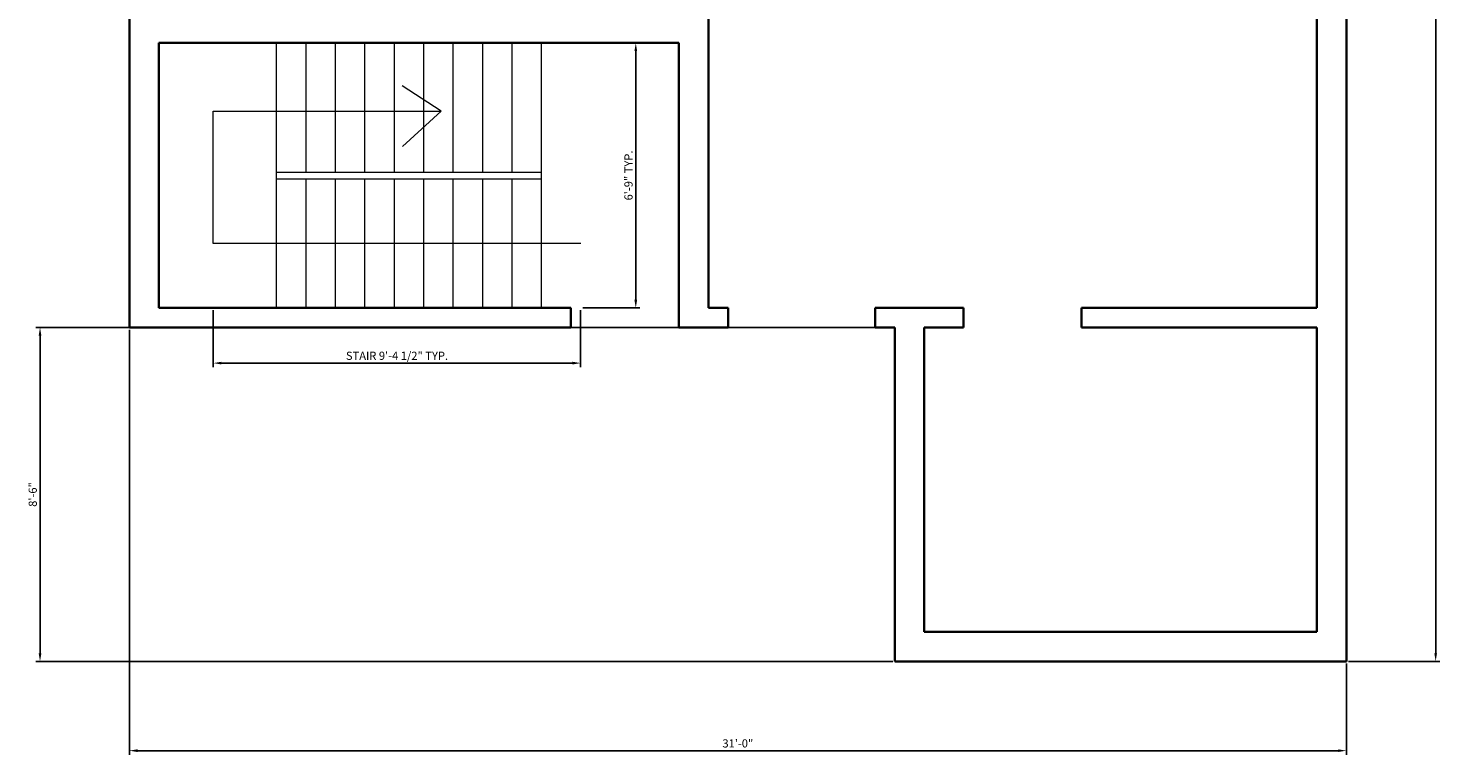
# Model space of a CAD drawing. Units: inches. Extents: x 2163 to 7246, y 928 to 2098.
# Tile 14 of 15: x 6815 to 7246, y 1403 to 1625. Entities that reach past the tile are written whole.
import ezdxf

# ---------------------------------------------------------------- set-up
doc = ezdxf.new("R2010")
doc.units = ezdxf.units.IN
for name, color, linetype, lineweight in [('A-ANNO-DIMS', 4, 'Continuous', 18), ('A-FLOR-STRS', 7, 'Continuous', 20), ('A-WALL', 7, 'Continuous', 35)]:
    doc.layers.add(name, color=color, linetype=linetype, lineweight=lineweight)
doc.styles.get("Standard").update_dxf_attribs({"font": 'arial.ttf'})
doc.dimstyles.new('ISO-25', dxfattribs={"dimtxt": 2.5, "dimasz": 2.5, "dimexe": 1.25, "dimexo": 0.625, "dimtad": 1, "dimdec": 0, "dimlunit": 3, "dimtxsty": 'Standard', "dimcen": 2.5, "dimadec": 0, "dimazin": 0, "dimtfac": 1, "dimtdec": 0, "dimtmove": 0, "dimatfit": 3, "dimfxl": 1, "dimarcsym": 0})

# ---------------------------------------------------------------- blocks, each defined once
blk = doc.blocks.new('STAIR-DOGLEG-81')
for p, q in [((19.35, 0), (19.35, 81)), ((28.35, 41.5), (28.35, 81)), ((37.35, 41.5), (37.35, 81)), ((46.35, 41.5), (46.35, 81)), ((55.35, 41.5), (55.35, 81)), ((64.35, 41.5), (64.35, 81)), ((73.35, 41.5), (73.35, 81)), ((82.35, 41.5), (82.35, 81)), ((91.35, 41.5), (91.35, 81)), ((100.35, 0), (100.35, 81)), ((69.69, 60.16), (57.76, 67.88)), ((0, 19.75), (0, 60.16)), ((0, 60.16), (69.69, 60.16)), ((69.69, 60.16), (57.82, 49.34)), ((19.35, 41.5), (100.35, 41.5)), ((19.35, 39.5), (100.35, 39.5)), ((28.35, 0), (28.35, 39.5)), ((37.35, 0), (37.35, 39.5)), ((46.35, 0), (46.35, 39.5)), ((55.35, 0), (55.35, 39.5)), ((64.35, 0), (64.35, 39.5)), ((73.35, 0), (73.35, 39.5)), ((82.35, 0), (82.35, 39.5)), ((91.35, 0), (91.35, 39.5)), ((112.3, 19.75), (0, 19.75))]:
    blk.add_line(p, q)
blk = doc.blocks.new('*D69')
at = {"layer": 'A-ANNO-DIMS', "color": 0, "lineweight": -2, "transparency": 16777216}
for p, q in [((6871.12, 1538.83), (6871.12, 1521.36)), ((6983.41, 1538.83), (6983.41, 1521.36)), ((6873.62, 1522.61), (6980.91, 1522.61))]:
    blk.add_line(p, q, dxfattribs=at)
at = {"layer": 'A-ANNO-DIMS', "color": 0, "transparency": 16777216}
for points in [[(6873.62, 1523.03), (6873.62, 1522.2), (6871.12, 1522.61)], [(6980.91, 1523.03), (6980.91, 1522.2), (6983.41, 1522.61)]]:
    blk.add_solid(points, dxfattribs=at)
at = {"layer": 'Defpoints', "color": 0, "transparency": 16777216}
for p in [(6871.12, 1539.46), (6983.41, 1539.46), (6983.41, 1522.61)]:
    blk.add_point(p, dxfattribs=at)
at = {"layer": 'A-ANNO-DIMS', "color": 0, "transparency": 16777216, "insert": (6927.27, 1524.53), "char_height": 2.5, "attachment_point": 5}
blk.add_mtext('STAIR 9\'-4 1/2" TYP.', dxfattribs=at)
blk = doc.blocks.new('*D70')
at = {"layer": 'A-ANNO-DIMS', "color": 0, "lineweight": -2, "transparency": 16777216}
for p, q in [((6984.04, 1620.46), (7001.51, 1620.46)), ((7000.26, 1541.96), (7000.26, 1617.96)), ((6984.04, 1539.46), (7001.51, 1539.46))]:
    blk.add_line(p, q, dxfattribs=at)
at = {"layer": 'A-ANNO-DIMS', "color": 0, "transparency": 16777216}
for points in [[(6999.84, 1617.96), (7000.68, 1617.96), (7000.26, 1620.46)], [(6999.84, 1541.96), (7000.68, 1541.96), (7000.26, 1539.46)]]:
    blk.add_solid(points, dxfattribs=at)
at = {"layer": 'Defpoints', "color": 0, "transparency": 16777216}
for p in [(6983.41, 1620.46), (7000.26, 1620.46), (6983.41, 1539.46)]:
    blk.add_point(p, dxfattribs=at)
at = {"layer": 'A-ANNO-DIMS', "color": 0, "transparency": 16777216, "insert": (6998.36, 1579.96), "char_height": 2.5, "attachment_point": 5, "rotation": 90}
blk.add_mtext('6\'-9" TYP.', dxfattribs=at)
blk = doc.blocks.new('*D112')
at = {"layer": 'A-ANNO-DIMS', "color": 0, "lineweight": -2, "transparency": 16777216}
for p, q in [((6845.46, 1532.83), (6845.46, 1402.91)), ((7217.46, 1430.83), (7217.46, 1402.91)), ((6847.96, 1404.16), (7214.96, 1404.16))]:
    blk.add_line(p, q, dxfattribs=at)
at = {"layer": 'A-ANNO-DIMS', "color": 0, "transparency": 16777216}
for points in [[(6847.96, 1404.58), (6847.96, 1403.74), (6845.46, 1404.16)], [(7214.96, 1404.58), (7214.96, 1403.74), (7217.46, 1404.16)]]:
    blk.add_solid(points, dxfattribs=at)
at = {"layer": 'Defpoints', "color": 0, "transparency": 16777216}
for p in [(6845.46, 1533.46), (7217.46, 1431.46), (7217.46, 1404.16)]:
    blk.add_point(p, dxfattribs=at)
at = {"layer": 'A-ANNO-DIMS', "color": 0, "transparency": 16777216, "insert": (7031.46, 1406.06), "char_height": 2.5, "attachment_point": 5}
blk.add_mtext('31\'-0"', dxfattribs=at)
blk = doc.blocks.new('*D113')
at = {"layer": 'A-ANNO-DIMS', "color": 0, "lineweight": -2, "transparency": 16777216}
for p, q in [((7218.09, 1974.46), (7246.01, 1974.46)), ((7244.76, 1971.96), (7244.76, 1433.96)), ((7218.09, 1431.46), (7246.01, 1431.46))]:
    blk.add_line(p, q, dxfattribs=at)
at = {"layer": 'A-ANNO-DIMS', "color": 0, "transparency": 16777216}
for points in [[(7244.34, 1971.96), (7245.18, 1971.96), (7244.76, 1974.46)], [(7244.34, 1433.96), (7245.18, 1433.96), (7244.76, 1431.46)]]:
    blk.add_solid(points, dxfattribs=at)
at = {"layer": 'Defpoints', "color": 0, "transparency": 16777216}
for p in [(7217.46, 1974.46), (7217.46, 1431.46), (7244.76, 1431.46)]:
    blk.add_point(p, dxfattribs=at)
at = {"layer": 'A-ANNO-DIMS', "color": 0, "transparency": 16777216, "insert": (7242.86, 1702.96), "char_height": 2.5, "attachment_point": 5, "rotation": 90}
blk.add_mtext('45\'-3"', dxfattribs=at)
blk = doc.blocks.new('*D114')
at = {"layer": 'A-ANNO-DIMS', "color": 0, "lineweight": -2, "transparency": 16777216}
for p, q in [((7078.84, 1533.46), (6816.91, 1533.46)), ((6818.16, 1530.96), (6818.16, 1433.96)), ((7078.84, 1431.46), (6816.91, 1431.46))]:
    blk.add_line(p, q, dxfattribs=at)
at = {"layer": 'A-ANNO-DIMS', "color": 0, "transparency": 16777216}
for points in [[(6817.74, 1530.96), (6818.58, 1530.96), (6818.16, 1533.46)], [(6817.74, 1433.96), (6818.58, 1433.96), (6818.16, 1431.46)]]:
    blk.add_solid(points, dxfattribs=at)
at = {"layer": 'Defpoints', "color": 0, "transparency": 16777216}
for p in [(7079.46, 1533.46), (6818.16, 1431.46), (7079.46, 1431.46)]:
    blk.add_point(p, dxfattribs=at)
at = {"layer": 'A-ANNO-DIMS', "color": 0, "transparency": 16777216, "insert": (6816.26, 1482.46), "char_height": 2.5, "attachment_point": 5, "rotation": 90}
blk.add_mtext('8\'-6"', dxfattribs=at)

msp = doc.modelspace()

# ---------------------------------------------------------------- linework, layer by layer
at = {"layer": 'A-WALL'}
for p, q in [((6845.46, 1533.46), (6845.46, 1974.46)), ((7217.46, 1974.46), (7217.46, 1431.46)), ((7208.46, 1815.46), (7208.46, 1539.46)), ((7022.46, 1755.46), (7022.46, 1539.46)), ((6854.46, 1620.46), (7013.46, 1620.46)), ((6854.46, 1539.46), (6854.46, 1620.46)), ((7013.46, 1620.46), (7013.46, 1533.46)), ((6854.46, 1539.46), (6980.46, 1539.46)), ((6980.46, 1533.46), (6980.46, 1539.46)), ((7022.46, 1539.46), (7028.46, 1539.46)), ((7028.46, 1539.46), (7028.46, 1533.46)), ((7073.46, 1539.46), (7100.46, 1539.46)), ((7073.46, 1539.46), (7073.46, 1533.46)), ((7100.46, 1539.46), (7100.46, 1533.46)), ((7136.46, 1539.46), (7208.46, 1539.46)), ((7136.46, 1539.46), (7136.46, 1533.46)), ((6845.46, 1533.46), (6980.46, 1533.46)), ((7013.46, 1533.46), (7028.46, 1533.46)), ((7073.46, 1533.46), (7079.46, 1533.46)), ((7079.46, 1533.46), (7079.46, 1431.46)), ((7088.46, 1533.46), (7100.46, 1533.46)), ((7088.46, 1533.46), (7088.46, 1440.46)), ((7136.46, 1533.46), (7208.46, 1533.46)), ((7208.46, 1533.46), (7208.46, 1440.46)), ((7208.46, 1440.46), (7088.46, 1440.46)), ((7217.46, 1431.46), (7079.46, 1431.46))]:
    msp.add_line(p, q, dxfattribs=at)

# ---------------------------------------------------------------- block references
at = {"layer": 'A-FLOR-STRS'}
msp.add_blockref('STAIR-DOGLEG-81', (6871.12, 1539.46), dxfattribs=at)

# ---------------------------------------------------------------- dimensions: what is measured, and where the dimension line sits
at = {"layer": 'A-ANNO-DIMS'}
for base, p1, p2, picture, middle in [((7244.76, 1431.46), (7217.46, 1974.46), (7217.46, 1431.46), '*D113', (7242.86, 1702.96)), ((6818.16, 1431.46), (7079.46, 1533.46), (7079.46, 1431.46), '*D114', (6816.26, 1482.46))]:
    dim = msp.add_linear_dim(base=base, p1=p1, p2=p2, angle=90, dimstyle='ISO-25', override={"dimdec": 1, "dimlfac": 1, "dimrnd": 0, "dimzin": 1, "dimdsep": 46, "dimlunit": 4, "dimfrac": 2}, dxfattribs=at)
    dim.commit()
    dim.dimension.update_dxf_attribs({"geometry": picture, "text_midpoint": middle})
dim = msp.add_linear_dim(base=(7000.26, 1620.46), p1=(6983.41, 1539.46), p2=(6983.41, 1620.46), angle=90, text='<> TYP.', dimstyle='ISO-25', override={"dimdec": 1, "dimlfac": 1, "dimrnd": 0, "dimzin": 1, "dimdsep": 46, "dimlunit": 4, "dimfrac": 2}, dxfattribs=at)
dim.commit()
dim.dimension.update_dxf_attribs({"geometry": '*D70', "text_midpoint": (6998.36, 1579.96)})
dim = msp.add_linear_dim(base=(6983.41, 1522.61), p1=(6871.12, 1539.46), p2=(6983.41, 1539.46), text='STAIR <> TYP.', dimstyle='ISO-25', override={"dimdec": 1, "dimlfac": 1, "dimrnd": 0, "dimzin": 1, "dimdsep": 46, "dimlunit": 4, "dimfrac": 2}, dxfattribs=at)
dim.commit()
dim.dimension.update_dxf_attribs({"geometry": '*D69', "text_midpoint": (6927.27, 1524.53)})
dim = msp.add_linear_dim(base=(7217.46, 1404.16), p1=(6845.46, 1533.46), p2=(7217.46, 1431.46), dimstyle='ISO-25', override={"dimdec": 1, "dimlfac": 1, "dimrnd": 0, "dimzin": 1, "dimdsep": 46, "dimlunit": 4, "dimfrac": 2}, dxfattribs=at)
dim.commit()
dim.dimension.update_dxf_attribs({"geometry": '*D112', "text_midpoint": (7031.46, 1406.06)})

doc.saveas('drawing.dxf')
